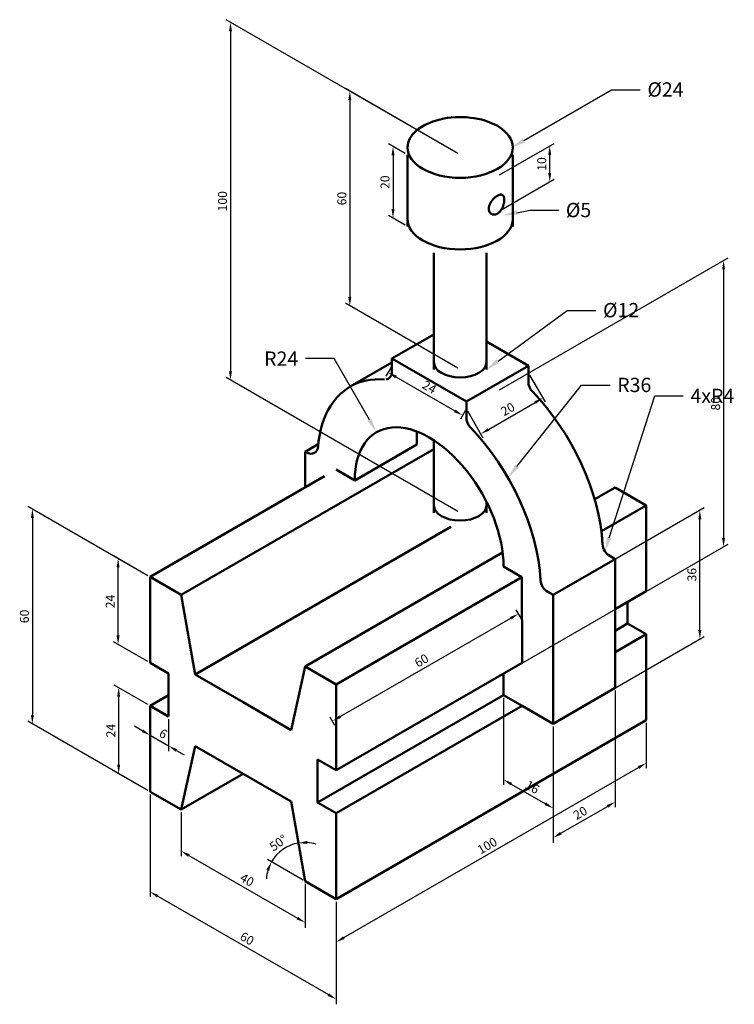
# Model space of a CAD drawing. Units: millimetres. Extents: x 2710 to 2910, y 851 to 1126.
import ezdxf
from ezdxf import colors
from ezdxf.entities.mleader import LeaderData, LeaderLine
from ezdxf.math import Vec2, Vec3

# ---------------------------------------------------------------- set-up
doc = ezdxf.new("R2010")
doc.units = ezdxf.units.MM
for name, color, linetype, lineweight in [('M-DIMS', 2, 'Continuous', 25), ('M-OUTL', 7, 'Continuous', 50), ('M-TEXT', 3, 'Continuous', 25)]:
    doc.layers.add(name, color=color, linetype=linetype, lineweight=lineweight)
doc.styles.get("Standard").update_dxf_attribs({"font": 'arial.ttf'})
doc.dimstyles.new('ISO-25', dxfattribs={"dimtxt": 2.5, "dimasz": 2.5, "dimexe": 1.25, "dimexo": 0.625, "dimtad": 1, "dimtxsty": 'Standard', "dimcen": 2.5, "dimadec": 0, "dimazin": 0, "dimtfac": 1, "dimtmove": 0, "dimatfit": 3, "dimfxl": 1, "dimarcsym": 0})

# ---------------------------------------------------------------- blocks, each defined once
blk = doc.blocks.new('*D1')
at = {"layer": 'Defpoints', "color": 0, "transparency": 16777216}
for p in [(2786.12, 907.33), (2785.15, 894.79), (2790.02, 885.08), (2790.02, 885.08), (2798.68, 880.08)]:
    blk.add_point(p, dxfattribs=at)
at = {"layer": 'M-DIMS', "color": 0, "lineweight": -2, "transparency": 16777216}
blk.add_line((2789.47, 885.4), (2779.53, 891.14), dxfattribs=at)
for start, end in [(99.9347, 150), (73.4842, 86.7094), (163.2252, 176.4505)]:
    blk.add_arc((2790.02, 885.08), 10.85, start, end, dxfattribs=at)
at = {"layer": 'M-DIMS', "color": 0, "transparency": 16777216}
for points in [[(2790.66, 895.5), (2790.61, 896.34), (2788.14, 895.78)], [(2779.24, 888.38), (2780.01, 888.05), (2780.62, 890.51)]]:
    blk.add_solid(points, dxfattribs=at)
at = {"layer": 'M-DIMS', "color": 0, "transparency": 16777216, "insert": (2782.71, 895.54), "char_height": 2.5, "attachment_point": 5, "rotation": 34.9673}
blk.add_mtext('50°', dxfattribs=at)
blk = doc.blocks.new('*D2')
at = {"layer": 'Defpoints', "color": 0, "transparency": 16777216}
for p in [(2885.28, 930.08), (2885.28, 918.09), (2798.68, 880.08)]:
    blk.add_point(p, dxfattribs=at)
at = {"layer": 'M-DIMS', "color": 0, "lineweight": -2, "transparency": 16777216}
for p, q in [((2885.28, 929.36), (2885.28, 916.65)), ((2800.84, 869.34), (2883.11, 916.84)), ((2798.68, 879.36), (2798.68, 866.65))]:
    blk.add_line(p, q, dxfattribs=at)
at = {"layer": 'M-DIMS', "color": 0, "transparency": 16777216}
for points in [[(2882.91, 917.2), (2883.32, 916.48), (2885.28, 918.09)], [(2800.63, 869.7), (2801.05, 868.98), (2798.68, 868.09)]]:
    blk.add_solid(points, dxfattribs=at)
at = {"layer": 'M-DIMS', "color": 0, "transparency": 16777216, "insert": (2841.03, 894.74), "char_height": 2.5, "attachment_point": 5, "rotation": 30}
blk.add_mtext('100', dxfattribs=at)
blk = doc.blocks.new('*D3')
at = {"layer": 'Defpoints', "color": 0, "transparency": 16777216}
for p in [(2737.95, 939.15), (2746.71, 934.08), (2746.71, 910.08)]:
    blk.add_point(p, dxfattribs=at)
at = {"layer": 'M-DIMS', "color": 0, "lineweight": -2, "transparency": 16777216}
for p, q in [((2746.09, 934.44), (2736.7, 939.87)), ((2737.95, 917.65), (2737.95, 936.65)), ((2746.09, 910.44), (2736.7, 915.87))]:
    blk.add_line(p, q, dxfattribs=at)
at = {"layer": 'M-DIMS', "color": 0, "transparency": 16777216}
for points in [[(2737.53, 936.65), (2738.36, 936.65), (2737.95, 939.15)], [(2737.53, 917.65), (2738.36, 917.65), (2737.95, 915.15)]]:
    blk.add_solid(points, dxfattribs=at)
at = {"layer": 'M-DIMS', "color": 0, "transparency": 16777216, "insert": (2736.07, 927.15), "char_height": 2.5, "attachment_point": 5, "rotation": 90}
blk.add_mtext('24', dxfattribs=at)
blk = doc.blocks.new('*D4')
at = {"layer": 'Defpoints', "color": 0, "transparency": 16777216}
for p in [(2737.78, 975.24), (2746.71, 970.08), (2746.71, 946.08)]:
    blk.add_point(p, dxfattribs=at)
at = {"layer": 'M-DIMS', "color": 0, "lineweight": -2, "transparency": 16777216}
for p, q in [((2746.09, 970.44), (2736.53, 975.96)), ((2737.78, 953.74), (2737.78, 972.74)), ((2746.09, 946.44), (2736.53, 951.96))]:
    blk.add_line(p, q, dxfattribs=at)
at = {"layer": 'M-DIMS', "color": 0, "transparency": 16777216}
for points in [[(2737.37, 972.74), (2738.2, 972.74), (2737.78, 975.24)], [(2737.37, 953.74), (2738.2, 953.74), (2737.78, 951.24)]]:
    blk.add_solid(points, dxfattribs=at)
at = {"layer": 'M-DIMS', "color": 0, "transparency": 16777216, "insert": (2735.9, 963.24), "char_height": 2.5, "attachment_point": 5, "rotation": 90}
blk.add_mtext('24', dxfattribs=at)
blk = doc.blocks.new('*D5')
at = {"layer": 'Defpoints', "color": 0, "transparency": 16777216}
for p in [(2746.71, 934.08), (2751.91, 931.08), (2751.91, 922.89)]:
    blk.add_point(p, dxfattribs=at)
at = {"layer": 'M-DIMS', "color": 0, "lineweight": -2, "transparency": 16777216}
for p, q in [((2746.71, 933.36), (2746.71, 924.44)), ((2751.91, 930.36), (2751.91, 921.44)), ((2744.55, 927.14), (2742.38, 928.39)), ((2746.71, 925.89), (2751.91, 922.89)), ((2754.08, 921.64), (2756.24, 920.39))]:
    blk.add_line(p, q, dxfattribs=at)
at = {"layer": 'M-DIMS', "color": 0, "transparency": 16777216}
for points in [[(2744.76, 927.5), (2744.34, 926.78), (2746.71, 925.89)], [(2754.28, 922), (2753.87, 921.28), (2751.91, 922.89)]]:
    blk.add_solid(points, dxfattribs=at)
at = {"layer": 'M-DIMS', "color": 0, "transparency": 16777216, "insert": (2750.26, 926.03), "char_height": 2.5, "attachment_point": 5, "rotation": 330}
blk.add_mtext('6', dxfattribs=at)
blk = doc.blocks.new('*D6')
at = {"layer": 'Defpoints', "color": 0, "transparency": 16777216}
for p in [(2849.63, 959.82), (2850.64, 958.08), (2798.68, 928.08)]:
    blk.add_point(p, dxfattribs=at)
at = {"layer": 'M-DIMS', "color": 0, "lineweight": -2, "transparency": 16777216}
for p, q in [((2850.33, 958.62), (2849.01, 960.91)), ((2799.84, 931.07), (2847.47, 958.57)), ((2798.36, 928.62), (2797.05, 930.91))]:
    blk.add_line(p, q, dxfattribs=at)
at = {"layer": 'M-DIMS', "color": 0, "transparency": 16777216}
for points in [[(2847.26, 958.93), (2847.68, 958.21), (2849.63, 959.82)], [(2799.63, 931.43), (2800.05, 930.71), (2797.67, 929.82)]]:
    blk.add_solid(points, dxfattribs=at)
at = {"layer": 'M-DIMS', "color": 0, "transparency": 16777216, "insert": (2822.7, 946.47), "char_height": 2.5, "attachment_point": 5, "rotation": 30}
blk.add_mtext('60', dxfattribs=at)
blk = doc.blocks.new('*D7')
at = {"layer": 'Defpoints', "color": 0, "transparency": 16777216}
for p in [(2876.62, 939.08), (2859.3, 929.08), (2876.62, 907.25)]:
    blk.add_point(p, dxfattribs=at)
at = {"layer": 'M-DIMS', "color": 0, "lineweight": -2, "transparency": 16777216}
for p, q in [((2876.62, 938.36), (2876.62, 905.8)), ((2859.3, 928.36), (2859.3, 895.8)), ((2861.46, 898.5), (2874.45, 906))]:
    blk.add_line(p, q, dxfattribs=at)
at = {"layer": 'M-DIMS', "color": 0, "transparency": 16777216}
for points in [[(2874.25, 906.36), (2874.66, 905.64), (2876.62, 907.25)], [(2861.25, 898.86), (2861.67, 898.14), (2859.3, 897.25)]]:
    blk.add_solid(points, dxfattribs=at)
at = {"layer": 'M-DIMS', "color": 0, "transparency": 16777216, "insert": (2867.01, 903.89), "char_height": 2.5, "attachment_point": 5, "rotation": 30}
blk.add_mtext('20', dxfattribs=at)
blk = doc.blocks.new('*D8')
at = {"layer": 'Defpoints', "color": 0, "transparency": 16777216}
for p in [(2900.26, 988.73), (2859.3, 965.08), (2859.3, 929.08)]:
    blk.add_point(p, dxfattribs=at)
at = {"layer": 'M-DIMS', "color": 0, "lineweight": -2, "transparency": 16777216}
for p, q in [((2859.92, 965.44), (2901.51, 989.46)), ((2900.26, 955.23), (2900.26, 986.23)), ((2859.92, 929.44), (2901.51, 953.46))]:
    blk.add_line(p, q, dxfattribs=at)
at = {"layer": 'M-DIMS', "color": 0, "transparency": 16777216}
for points in [[(2899.85, 986.23), (2900.68, 986.23), (2900.26, 988.73)], [(2899.85, 955.23), (2900.68, 955.23), (2900.26, 952.73)]]:
    blk.add_solid(points, dxfattribs=at)
at = {"layer": 'M-DIMS', "color": 0, "transparency": 16777216, "insert": (2898.36, 970.73), "char_height": 2.5, "attachment_point": 5, "rotation": 90}
blk.add_mtext('36', dxfattribs=at)
blk = doc.blocks.new('*D9')
at = {"layer": 'Defpoints', "color": 0, "transparency": 16777216}
for p in [(2833.32, 1088.02), (2769.18, 1025.06), (2833.32, 988.02)]:
    blk.add_point(p, dxfattribs=at)
at = {"layer": 'M-DIMS', "color": 0, "lineweight": -2, "transparency": 16777216}
for p, q in [((2832.69, 1088.39), (2767.93, 1125.78)), ((2769.18, 1122.56), (2769.18, 1027.56)), ((2832.69, 988.39), (2767.93, 1025.78))]:
    blk.add_line(p, q, dxfattribs=at)
at = {"layer": 'M-DIMS', "color": 0, "transparency": 16777216}
for points in [[(2768.76, 1122.56), (2769.59, 1122.56), (2769.18, 1125.06)], [(2768.76, 1027.56), (2769.59, 1027.56), (2769.18, 1025.06)]]:
    blk.add_solid(points, dxfattribs=at)
at = {"layer": 'M-DIMS', "color": 0, "transparency": 16777216, "insert": (2767.27, 1075.06), "char_height": 2.5, "attachment_point": 5, "rotation": 90}
blk.add_mtext('100', dxfattribs=at)
blk = doc.blocks.new('*D10')
at = {"layer": 'Defpoints', "color": 0, "transparency": 16777216}
for p in [(2833.32, 1088.02), (2802.51, 1045.81), (2833.32, 1028.02)]:
    blk.add_point(p, dxfattribs=at)
at = {"layer": 'M-DIMS', "color": 0, "lineweight": -2, "transparency": 16777216}
for p, q in [((2832.69, 1088.39), (2801.26, 1106.54)), ((2802.51, 1103.31), (2802.51, 1048.31)), ((2832.69, 1028.39), (2801.26, 1046.54))]:
    blk.add_line(p, q, dxfattribs=at)
at = {"layer": 'M-DIMS', "color": 0, "transparency": 16777216}
for points in [[(2802.09, 1103.31), (2802.92, 1103.31), (2802.51, 1105.81)], [(2802.09, 1048.31), (2802.92, 1048.31), (2802.51, 1045.81)]]:
    blk.add_solid(points, dxfattribs=at)
at = {"layer": 'M-DIMS', "color": 0, "transparency": 16777216, "insert": (2800.6, 1075.81), "char_height": 2.5, "attachment_point": 5, "rotation": 90}
blk.add_mtext('60', dxfattribs=at)
blk = doc.blocks.new('*D11')
at = {"layer": 'Defpoints', "color": 0, "transparency": 16777216}
for p in [(2852.37, 1027.02), (2856.39, 1020.06), (2835.05, 1017.02)]:
    blk.add_point(p, dxfattribs=at)
at = {"layer": 'M-DIMS', "color": 0, "lineweight": -2, "transparency": 16777216}
for p, q in [((2852.68, 1026.48), (2857.02, 1018.98)), ((2841.24, 1011.31), (2854.23, 1018.81)), ((2835.36, 1016.48), (2839.7, 1008.98))]:
    blk.add_line(p, q, dxfattribs=at)
at = {"layer": 'M-DIMS', "color": 0, "transparency": 16777216}
for points in [[(2854.02, 1019.17), (2854.44, 1018.45), (2856.39, 1020.06)], [(2841.03, 1011.67), (2841.45, 1010.95), (2839.07, 1010.06)]]:
    blk.add_solid(points, dxfattribs=at)
at = {"layer": 'M-DIMS', "color": 0, "transparency": 16777216, "insert": (2846.78, 1016.7), "char_height": 2.5, "attachment_point": 5, "rotation": 30}
blk.add_mtext('20', dxfattribs=at)
blk = doc.blocks.new('*D12')
at = {"layer": 'Defpoints', "color": 0, "transparency": 16777216}
for p in [(2814.26, 1029.02), (2834.01, 1015.23), (2835.05, 1017.02)]:
    blk.add_point(p, dxfattribs=at)
at = {"layer": 'M-DIMS', "color": 0, "lineweight": -2, "transparency": 16777216}
for p, q in [((2813.95, 1028.48), (2812.61, 1026.15)), ((2815.4, 1025.98), (2831.85, 1016.48)), ((2834.74, 1016.48), (2833.39, 1014.15))]:
    blk.add_line(p, q, dxfattribs=at)
at = {"layer": 'M-DIMS', "color": 0, "transparency": 16777216}
for points in [[(2815.6, 1026.34), (2815.19, 1025.62), (2813.23, 1027.23)], [(2832.06, 1016.84), (2831.64, 1016.12), (2834.01, 1015.23)]]:
    blk.add_solid(points, dxfattribs=at)
at = {"layer": 'M-DIMS', "color": 0, "transparency": 16777216, "insert": (2824.56, 1022.86), "char_height": 2.5, "attachment_point": 5, "rotation": 330}
blk.add_mtext('24', dxfattribs=at)
blk = doc.blocks.new('*D13')
at = {"layer": 'Defpoints', "color": 0, "transparency": 16777216}
for p in [(2843.71, 1022.02), (2906.89, 978.5), (2843.71, 942.02)]:
    blk.add_point(p, dxfattribs=at)
at = {"layer": 'M-DIMS', "color": 0, "lineweight": -2, "transparency": 16777216}
for p, q in [((2844.33, 1022.39), (2908.14, 1059.22)), ((2906.89, 1056), (2906.89, 981)), ((2844.33, 942.39), (2908.14, 979.22))]:
    blk.add_line(p, q, dxfattribs=at)
at = {"layer": 'M-DIMS', "color": 0, "transparency": 16777216}
for points in [[(2906.47, 1056), (2907.3, 1056), (2906.89, 1058.5)], [(2906.47, 981), (2907.3, 981), (2906.89, 978.5)]]:
    blk.add_solid(points, dxfattribs=at)
at = {"layer": 'M-DIMS', "color": 0, "transparency": 16777216, "insert": (2904.99, 1018.5), "char_height": 2.5, "attachment_point": 5, "rotation": 90}
blk.add_mtext('80', dxfattribs=at)
blk = doc.blocks.new('*D14')
at = {"layer": 'Defpoints', "color": 0, "transparency": 16777216}
for p in [(2845.44, 937.08), (2859.3, 929.08), (2859.3, 905.47)]:
    blk.add_point(p, dxfattribs=at)
at = {"layer": 'M-DIMS', "color": 0, "lineweight": -2, "transparency": 16777216}
for p, q in [((2845.44, 936.36), (2845.44, 912.03)), ((2859.3, 928.36), (2859.3, 904.03)), ((2847.61, 912.22), (2857.13, 906.72))]:
    blk.add_line(p, q, dxfattribs=at)
at = {"layer": 'M-DIMS', "color": 0, "transparency": 16777216}
for points in [[(2847.81, 912.58), (2847.4, 911.86), (2845.44, 913.47)], [(2857.34, 907.08), (2856.92, 906.36), (2859.3, 905.47)]]:
    blk.add_solid(points, dxfattribs=at)
at = {"layer": 'M-DIMS', "color": 0, "transparency": 16777216, "insert": (2853.32, 911.12), "char_height": 2.5, "attachment_point": 5, "rotation": 330}
blk.add_mtext('16', dxfattribs=at)
blk = doc.blocks.new('*D15')
at = {"layer": 'Defpoints', "color": 0, "transparency": 16777216}
for p in [(2746.71, 970.08), (2713.85, 929.06), (2746.71, 910.08)]:
    blk.add_point(p, dxfattribs=at)
at = {"layer": 'M-DIMS', "color": 0, "lineweight": -2, "transparency": 16777216}
for p, q in [((2746.09, 970.44), (2712.6, 989.78)), ((2713.85, 986.56), (2713.85, 931.56)), ((2746.09, 910.44), (2712.6, 929.78))]:
    blk.add_line(p, q, dxfattribs=at)
at = {"layer": 'M-DIMS', "color": 0, "transparency": 16777216}
for points in [[(2713.43, 986.56), (2714.27, 986.56), (2713.85, 989.06)], [(2713.43, 931.56), (2714.27, 931.56), (2713.85, 929.06)]]:
    blk.add_solid(points, dxfattribs=at)
at = {"layer": 'M-DIMS', "color": 0, "transparency": 16777216, "insert": (2711.95, 959.06), "char_height": 2.5, "attachment_point": 5, "rotation": 90}
blk.add_mtext('60', dxfattribs=at)
blk = doc.blocks.new('*D16')
at = {"layer": 'Defpoints', "color": 0, "transparency": 16777216}
for p in [(2746.71, 910.08), (2798.68, 880.08), (2798.68, 852.15)]:
    blk.add_point(p, dxfattribs=at)
at = {"layer": 'M-DIMS', "color": 0, "lineweight": -2, "transparency": 16777216}
for p, q in [((2746.71, 909.36), (2746.71, 880.7)), ((2748.88, 880.9), (2796.51, 853.4)), ((2798.68, 879.36), (2798.68, 850.7))]:
    blk.add_line(p, q, dxfattribs=at)
at = {"layer": 'M-DIMS', "color": 0, "transparency": 16777216}
for points in [[(2749.09, 881.26), (2748.67, 880.54), (2746.71, 882.15)], [(2796.72, 853.76), (2796.3, 853.04), (2798.68, 852.15)]]:
    blk.add_solid(points, dxfattribs=at)
at = {"layer": 'M-DIMS', "color": 0, "transparency": 16777216, "insert": (2773.65, 868.79), "char_height": 2.5, "attachment_point": 5, "rotation": 330}
blk.add_mtext('60', dxfattribs=at)
blk = doc.blocks.new('*D17')
at = {"layer": 'Defpoints', "color": 0, "transparency": 16777216}
for p in [(2755.37, 905.08), (2790.02, 885.08), (2790.02, 873.54)]:
    blk.add_point(p, dxfattribs=at)
at = {"layer": 'M-DIMS', "color": 0, "lineweight": -2, "transparency": 16777216}
for p, q in [((2755.37, 904.36), (2755.37, 892.1)), ((2757.54, 892.29), (2787.85, 874.79)), ((2790.02, 884.36), (2790.02, 872.1))]:
    blk.add_line(p, q, dxfattribs=at)
at = {"layer": 'M-DIMS', "color": 0, "transparency": 16777216}
for points in [[(2757.75, 892.65), (2757.33, 891.93), (2755.37, 893.54)], [(2788.06, 875.15), (2787.64, 874.43), (2790.02, 873.54)]]:
    blk.add_solid(points, dxfattribs=at)
at = {"layer": 'M-DIMS', "color": 0, "transparency": 16777216, "insert": (2773.65, 885.19), "char_height": 2.5, "attachment_point": 5, "rotation": 330}
blk.add_mtext('40', dxfattribs=at)
blk = doc.blocks.new('*D18')
at = {"layer": 'Defpoints', "color": 0, "transparency": 16777216}
for p in [(2818.62, 1088.02), (2814.57, 1070.37), (2818.62, 1068.02)]:
    blk.add_point(p, dxfattribs=at)
at = {"layer": 'M-DIMS', "color": 0, "lineweight": -2, "transparency": 16777216}
for p, q in [((2818, 1088.39), (2813.32, 1091.09)), ((2814.57, 1087.87), (2814.57, 1072.87)), ((2818, 1068.39), (2813.32, 1071.09))]:
    blk.add_line(p, q, dxfattribs=at)
at = {"layer": 'M-DIMS', "color": 0, "transparency": 16777216}
for points in [[(2814.15, 1087.87), (2814.98, 1087.87), (2814.57, 1090.37)], [(2814.15, 1072.87), (2814.98, 1072.87), (2814.57, 1070.37)]]:
    blk.add_solid(points, dxfattribs=at)
at = {"layer": 'M-DIMS', "color": 0, "transparency": 16777216, "insert": (2812.66, 1080.37), "char_height": 2.5, "attachment_point": 5, "rotation": 90}
blk.add_mtext('20', dxfattribs=at)
blk = doc.blocks.new('*D19')
at = {"layer": 'Defpoints', "color": 0, "transparency": 16777216}
for p in [(2858.34, 1090.47), (2843.71, 1082.02), (2843.71, 1072.02)]:
    blk.add_point(p, dxfattribs=at)
at = {"layer": 'M-DIMS', "color": 0, "lineweight": -2, "transparency": 16777216}
for p, q in [((2844.33, 1082.39), (2859.59, 1091.19)), ((2858.34, 1082.97), (2858.34, 1087.97)), ((2844.33, 1072.39), (2859.59, 1081.19))]:
    blk.add_line(p, q, dxfattribs=at)
at = {"layer": 'M-DIMS', "color": 0, "transparency": 16777216}
for points in [[(2857.92, 1087.97), (2858.75, 1087.97), (2858.34, 1090.47)], [(2857.92, 1082.97), (2858.75, 1082.97), (2858.34, 1080.47)]]:
    blk.add_solid(points, dxfattribs=at)
at = {"layer": 'M-DIMS', "color": 0, "transparency": 16777216, "insert": (2856.43, 1085.47), "char_height": 2.5, "attachment_point": 5, "rotation": 90}
blk.add_mtext('10', dxfattribs=at)

msp = doc.modelspace()

# ---------------------------------------------------------------- linework, layer by layer
at = {"layer": 'M-OUTL'}
for p, q in [((2818.62, 1088.025), (2818.62, 1068.025)), ((2848.014, 1088.025), (2848.014, 1068.025)), ((2825.969, 1060.676), (2825.969, 1028.025)), ((2840.666, 1060.676), (2840.666, 1028.025)), ((2814.265, 1031.084), (2825.969, 1037.841)), ((2852.37, 1029.084), (2840.666, 1035.841)), ((2814.265, 1029.995), (2802.612, 1023.267)), ((2835.049, 1019.084), (2814.265, 1031.084)), ((2814.265, 1027.744), (2814.265, 1031.084)), ((2814.265, 1027.075), (2814.265, 1029.025)), ((2835.049, 1019.084), (2852.37, 1029.084)), ((2852.37, 1025.744), (2852.37, 1029.084)), ((2852.37, 1024.669), (2852.37, 1027.025)), ((2835.049, 1015.744), (2835.049, 1019.084)), ((2835.049, 1014.669), (2835.049, 1017.025)), ((2821.193, 1007.084), (2821.193, 1010.748)), ((2790.016, 1005.084), (2793.698, 1007.21)), ((2803.872, 997.084), (2821.193, 1007.084)), ((2825.969, 988.025), (2825.969, 1008.278)), ((2755.375, 965.084), (2825.969, 1005.841)), ((2790.19, 1004.983), (2790.016, 1005.084)), ((2790.016, 995.084), (2790.016, 1005.084)), ((2798.676, 1000.084), (2803.872, 997.084)), ((2746.715, 970.084), (2795.462, 998.228)), ((2870.911, 991.788), (2876.619, 995.084)), ((2885.279, 990.084), (2876.619, 995.084)), ((2840.666, 988.025), (2840.666, 991.148)), ((2885.279, 990.084), (2872.779, 982.867)), ((2885.279, 990.084), (2885.279, 966.084)), ((2759.272, 942.834), (2830.685, 984.064)), ((2790.016, 945.084), (2845.192, 976.939)), ((2859.298, 965.084), (2876.619, 975.084)), ((2875.096, 975.963), (2876.619, 975.084)), ((2876.619, 975.084), (2876.619, 939.084)), ((2850.553, 970.034), (2845.441, 972.985)), ((2746.715, 946.084), (2746.715, 970.084)), ((2746.715, 970.084), (2755.375, 965.084)), ((2850.553, 970.034), (2798.676, 940.084)), ((2850.638, 946.084), (2850.553, 970.034)), ((2859.298, 965.084), (2857.775, 965.963)), ((2876.619, 961.084), (2885.279, 966.084)), ((2755.375, 965.084), (2759.272, 942.834)), ((2859.298, 929.084), (2859.298, 965.084)), ((2880.083, 963.084), (2880.083, 957.084)), ((2876.619, 955.084), (2880.083, 957.084)), ((2880.083, 957.084), (2885.279, 954.084)), ((2876.619, 949.084), (2885.279, 954.084)), ((2885.279, 954.084), (2885.279, 930.084)), ((2751.911, 943.084), (2746.715, 946.084)), ((2786.119, 927.334), (2790.016, 945.084)), ((2798.676, 940.084), (2790.016, 945.084)), ((2798.676, 916.084), (2850.638, 946.084)), ((2798.676, 916.084), (2850.638, 946.084)), ((2751.911, 931.084), (2751.911, 943.084)), ((2772.695, 935.084), (2759.272, 942.834)), ((2845.442, 937.084), (2845.442, 943.084)), ((2798.676, 940.084), (2798.676, 916.084)), ((2876.619, 939.084), (2859.298, 929.084)), ((2746.715, 934.084), (2751.911, 937.084)), ((2793.48, 907.084), (2845.442, 937.084)), ((2850.638, 934.084), (2845.442, 937.084)), ((2746.715, 910.084), (2746.715, 934.084)), ((2746.715, 934.084), (2751.911, 931.084)), ((2772.695, 935.084), (2786.119, 927.334)), ((2798.676, 904.084), (2850.638, 934.084)), ((2798.676, 904.084), (2850.638, 934.084)), ((2850.638, 934.084), (2859.298, 929.084)), ((2798.676, 880.084), (2885.279, 930.084)), ((2759.272, 922.834), (2755.375, 905.084)), ((2772.695, 915.084), (2759.272, 922.834)), ((2798.676, 916.084), (2793.48, 919.084)), ((2793.48, 919.084), (2793.48, 907.084)), ((2755.375, 905.084), (2772.695, 915.084)), ((2772.695, 915.084), (2786.119, 907.334)), ((2746.715, 910.084), (2755.375, 905.084)), ((2786.119, 907.334), (2790.016, 885.084)), ((2793.48, 907.084), (2798.676, 904.084)), ((2798.676, 904.084), (2798.676, 880.084)), ((2798.676, 880.084), (2790.016, 885.084))]:
    msp.add_line(p, q, dxfattribs=at)
for points in [[(2842.065, 1071.497), (2842.026, 1071.521), (2841.988, 1071.546), (2841.951, 1071.572), (2841.914, 1071.599), (2841.878, 1071.628), (2841.843, 1071.657), (2841.81, 1071.688), (2841.777, 1071.721), (2841.745, 1071.754), (2841.714, 1071.789), (2841.684, 1071.825), (2841.655, 1071.862), (2841.627, 1071.9), (2841.6, 1071.939), (2841.575, 1071.979), (2841.55, 1072.02), (2841.527, 1072.062), (2841.504, 1072.105), (2841.483, 1072.149), (2841.463, 1072.194), (2841.445, 1072.24), (2841.427, 1072.287), (2841.411, 1072.335), (2841.396, 1072.383), (2841.382, 1072.432), (2841.37, 1072.483), (2841.359, 1072.533), (2841.349, 1072.585), (2841.34, 1072.637), (2841.333, 1072.69), (2841.327, 1072.743), (2841.323, 1072.798), (2841.319, 1072.852), (2841.317, 1072.908), (2841.316, 1072.963), (2841.317, 1073.02), (2841.319, 1073.076), (2841.322, 1073.134), (2841.327, 1073.191), (2841.333, 1073.249), (2841.34, 1073.308), (2841.348, 1073.367), (2841.358, 1073.426), (2841.369, 1073.486), (2841.382, 1073.546), (2841.396, 1073.606), (2841.411, 1073.667), (2841.427, 1073.728), (2841.445, 1073.789), (2841.464, 1073.85), (2841.485, 1073.912), (2841.507, 1073.974), (2841.53, 1074.037), (2841.554, 1074.099), (2841.58, 1074.162), (2841.607, 1074.225), (2841.635, 1074.288), (2841.665, 1074.352), (2841.696, 1074.415), (2841.729, 1074.479), (2841.762, 1074.543), (2841.798, 1074.607), (2841.834, 1074.671), (2841.872, 1074.735), (2841.911, 1074.799), (2841.951, 1074.863), (2841.993, 1074.927), (2842.036, 1074.991), (2842.081, 1075.055), (2842.127, 1075.12), (2842.175, 1075.184), (2842.224, 1075.249), (2842.274, 1075.313), (2842.326, 1075.377), (2842.379, 1075.441), (2842.434, 1075.505), (2842.49, 1075.568), (2842.547, 1075.631), (2842.605, 1075.693), (2842.664, 1075.755), (2842.725, 1075.815), (2842.786, 1075.875), (2842.848, 1075.934), (2842.911, 1075.992), (2842.975, 1076.049), (2843.04, 1076.105), (2843.105, 1076.16), (2843.171, 1076.213), (2843.237, 1076.265), (2843.304, 1076.315), (2843.371, 1076.364), (2843.438, 1076.412), (2843.506, 1076.457), (2843.574, 1076.501), (2843.642, 1076.543), (2843.71, 1076.584)], [(2845.127, 1076.801), (2845.168, 1076.776), (2845.206, 1076.748), (2845.243, 1076.719), (2845.277, 1076.687), (2845.31, 1076.653), (2845.342, 1076.616), (2845.371, 1076.578), (2845.399, 1076.538), (2845.425, 1076.496), (2845.45, 1076.452), (2845.473, 1076.406), (2845.495, 1076.359), (2845.515, 1076.309), (2845.533, 1076.258), (2845.55, 1076.206), (2845.566, 1076.151), (2845.58, 1076.096), (2845.593, 1076.038), (2845.604, 1075.98), (2845.614, 1075.919), (2845.623, 1075.858), (2845.63, 1075.795), (2845.636, 1075.73), (2845.641, 1075.665), (2845.644, 1075.598), (2845.646, 1075.529), (2845.647, 1075.46), (2845.646, 1075.389), (2845.644, 1075.318), (2845.64, 1075.245), (2845.635, 1075.171), (2845.629, 1075.096), (2845.622, 1075.02), (2845.613, 1074.943), (2845.603, 1074.865), (2845.591, 1074.786), (2845.578, 1074.706), (2845.564, 1074.625), (2845.548, 1074.544), (2845.531, 1074.462), (2845.512, 1074.379), (2845.492, 1074.295), (2845.47, 1074.211), (2845.447, 1074.126), (2845.422, 1074.04), (2845.395, 1073.954), (2845.367, 1073.867), (2845.337, 1073.78), (2845.306, 1073.693), (2845.272, 1073.605), (2845.237, 1073.517), (2845.201, 1073.429), (2845.162, 1073.341), (2845.121, 1073.253), (2845.079, 1073.165), (2845.035, 1073.077), (2844.988, 1072.99), (2844.939, 1072.902), (2844.888, 1072.814), (2844.834, 1072.726), (2844.777, 1072.638), (2844.718, 1072.551), (2844.657, 1072.465), (2844.593, 1072.381), (2844.527, 1072.298), (2844.458, 1072.217), (2844.388, 1072.138), (2844.316, 1072.062), (2844.241, 1071.988), (2844.165, 1071.917), (2844.088, 1071.85), (2844.008, 1071.786), (2843.928, 1071.725), (2843.846, 1071.668), (2843.763, 1071.615), (2843.679, 1071.566), (2843.595, 1071.522), (2843.51, 1071.481), (2843.425, 1071.445), (2843.339, 1071.413), (2843.254, 1071.385), (2843.168, 1071.362), (2843.084, 1071.343), (2842.999, 1071.329), (2842.915, 1071.319), (2842.832, 1071.314), (2842.749, 1071.313), (2842.667, 1071.316), (2842.587, 1071.324), (2842.507, 1071.336), (2842.429, 1071.353), (2842.353, 1071.373), (2842.278, 1071.398), (2842.205, 1071.427), (2842.134, 1071.46), (2842.065, 1071.497)], [(2843.71, 1076.584), (2843.729, 1076.595), (2843.748, 1076.606), (2843.767, 1076.616), (2843.786, 1076.627), (2843.805, 1076.637), (2843.824, 1076.647), (2843.843, 1076.657), (2843.862, 1076.667), (2843.881, 1076.676), (2843.9, 1076.685), (2843.918, 1076.695), (2843.937, 1076.703), (2843.955, 1076.712), (2843.973, 1076.721), (2843.992, 1076.729), (2844.01, 1076.737), (2844.028, 1076.745), (2844.046, 1076.753), (2844.064, 1076.76), (2844.081, 1076.768), (2844.099, 1076.775), (2844.117, 1076.782), (2844.134, 1076.789), (2844.152, 1076.795), (2844.169, 1076.802), (2844.186, 1076.808), (2844.204, 1076.814), (2844.221, 1076.82), (2844.238, 1076.825), (2844.254, 1076.831), (2844.271, 1076.836), (2844.288, 1076.841), (2844.304, 1076.846), (2844.321, 1076.85), (2844.337, 1076.855), (2844.354, 1076.859), (2844.37, 1076.863), (2844.386, 1076.867), (2844.402, 1076.871), (2844.418, 1076.874), (2844.433, 1076.878), (2844.449, 1076.881), (2844.464, 1076.884), (2844.48, 1076.887), (2844.495, 1076.889), (2844.51, 1076.892), (2844.525, 1076.894), (2844.54, 1076.896), (2844.555, 1076.898), (2844.57, 1076.899), (2844.585, 1076.901), (2844.599, 1076.902), (2844.614, 1076.903), (2844.628, 1076.904), (2844.642, 1076.905), (2844.656, 1076.906), (2844.67, 1076.906), (2844.684, 1076.907), (2844.698, 1076.907), (2844.712, 1076.907), (2844.725, 1076.907), (2844.739, 1076.906), (2844.752, 1076.906), (2844.765, 1076.905), (2844.778, 1076.904), (2844.791, 1076.903), (2844.804, 1076.902), (2844.817, 1076.9), (2844.83, 1076.899), (2844.842, 1076.897), (2844.854, 1076.895), (2844.867, 1076.893), (2844.879, 1076.891), (2844.891, 1076.889), (2844.903, 1076.886), (2844.915, 1076.884), (2844.926, 1076.881), (2844.938, 1076.878), (2844.95, 1076.875), (2844.961, 1076.872), (2844.972, 1076.868), (2844.983, 1076.865), (2844.994, 1076.861), (2845.005, 1076.857), (2845.016, 1076.853), (2845.027, 1076.849), (2845.037, 1076.845), (2845.048, 1076.84), (2845.058, 1076.836), (2845.068, 1076.831), (2845.078, 1076.826), (2845.088, 1076.822), (2845.098, 1076.817), (2845.108, 1076.811), (2845.118, 1076.806), (2845.127, 1076.801)]]:
    msp.add_lwpolyline(points, dxfattribs=at)
for centre, start, end in [((2856.37, 1024.669), 180, 223.98051), ((2839.049, 1014.669), 180, 223.98051), ((2877.096, 979.427), 182.83372, 240), ((2859.775, 969.427), 182.83372, 240)]:
    msp.add_arc(centre, 4, start, end, dxfattribs=at)
for centre, major_axis, start_param, end_param in [((2833.317, 1090.084), (14.697, 0), 0.7853982, 3.1415927), ((2833.317, 1090.084), (14.697, 0), 0, 0.7853982), ((2833.317, 1090.084), (14.697, 0), 3.1415927, 6.2831853), ((2833.317, 1070.084), (14.697, 0), 3.1415927, 6.2831853), ((2833.317, 1030.084), (7.348, 0), 3.1415927, 6.2831853), ((2811.493, 1029.498), (1.531, -4.18), 6.1460382, 7.0428047), ((2824.657, 985.084), (-22.045, 38.184), 5.909304, 6.2831853), ((2824.657, 985.084), (-22.045, 38.184), 0, 0.6852307), ((2841.977, 995.084), (22.045, -38.184), 0.8441674, 1.9779262), ((2824.657, 985.084), (14.697, -25.456), 0.7813003, 3.9269908), ((2824.657, 985.084), (22.045, -38.184), 0.8441674, 1.9779262), ((2790.19, 1008.983), (2.449, -4.243), 5.4977871, 6.2831853), ((2790.19, 1008.983), (2.449, -4.243), 0, 0.6852307), ((2833.317, 990.084), (7.348, 0), 3.1415927, 6.2831853)]:
    msp.add_ellipse(centre, major_axis=major_axis, ratio=0.5773503, start_param=start_param, end_param=end_param, dxfattribs=at)

# ---------------------------------------------------------------- dimensions: what is measured, and where the dimension line sits
at = {"layer": 'M-DIMS'}
for p1, p2, distance, picture, middle in [((2833.317, 1088.025), (2833.317, 988.025), -64.141, '*D9', (2767.275, 1075.057)), ((2833.317, 1088.025), (2833.317, 1028.025), -30.812, '*D10', (2800.604, 1075.814)), ((2814.265, 1029.025), (2835.049, 1017.025), -2.069, '*D12', (2824.563, 1022.861)), ((2835.049, 1017.025), (2852.37, 1027.025), -8.045, '*D11', (2846.781, 1016.704)), ((2746.715, 970.084), (2746.715, 910.084), -32.866, '*D15', (2711.948, 959.059)), ((2859.298, 929.084), (2859.298, 965.084), -40.965, '*D8', (2898.36, 970.735)), ((2746.715, 946.084), (2746.715, 970.084), 8.93, '*D4', (2735.905, 963.239)), ((2798.676, 928.084), (2850.638, 958.084), 2.008, '*D6', (2822.702, 946.47)), ((2746.715, 910.084), (2746.715, 934.084), 8.768, '*D3', (2736.066, 927.146)), ((2859.298, 929.084), (2876.619, 939.084), -27.572, '*D7', (2867.008, 903.893)), ((2845.442, 937.084), (2859.298, 929.084), -20.448, '*D14', (2853.321, 911.119)), ((2746.715, 934.084), (2751.911, 931.084), -7.099, '*D5', (2750.263, 926.033)), ((2798.676, 880.084), (2885.279, 930.084), -10.385, '*D2', (2841.027, 894.739)), ((2746.715, 910.084), (2798.676, 880.084), -24.193, '*D16', (2773.646, 868.794)), ((2755.375, 905.084), (2790.016, 885.084), -9.994, '*D17', (2773.646, 885.19))]:
    dim = msp.add_aligned_dim(p1=p1, p2=p2, distance=distance, dimstyle='ISO-25', override={"dimclrd": 0, "dimclre": 0, "dimclrt": 0}, dxfattribs=at)
    dim.commit()
    dim.dimension.update_dxf_attribs({"geometry": picture, "text_midpoint": middle})
for base, p1, p2, picture, middle in [((2814.566, 1070.365), (2818.62, 1088.025), (2818.62, 1068.025), '*D18', (2812.665, 1080.365)), ((2858.335, 1090.469), (2843.71, 1072.025), (2843.71, 1082.025), '*D19', (2856.434, 1085.469)), ((2906.887, 978.5), (2843.71, 1022.025), (2843.71, 942.025), '*D13', (2904.986, 1018.5))]:
    dim = msp.add_linear_dim(base=base, p1=p1, p2=p2, angle=90, dimstyle='ISO-25', override={"dimclrd": 0, "dimclre": 0, "dimclrt": 0}, dxfattribs=at)
    dim.commit()
    dim.dimension.update_dxf_attribs({"geometry": picture, "text_midpoint": middle})
dim = msp.add_angular_dim_2l(base=(2785.152, 894.788), line1=((2786.119, 907.334), (2790.016, 885.084)), line2=((2798.676, 880.084), (2790.016, 885.084)), dimstyle='ISO-25', override={"dimclrd": 0, "dimclre": 0, "dimclrt": 0}, dxfattribs=at)
dim.commit()
dim.dimension.update_dxf_attribs({"geometry": '*D1', "text_midpoint": (2782.705, 895.537)})

# ---------------------------------------------------------------- leaders
at = {"layer": 'M-TEXT'}
ml = msp.add_multileader_mtext('Standard', dxfattribs=at)
ml.set_content('%%C24', color=256)
ml.set_leader_properties()
ml.build(insert=Vec2(0, 0))
ctx = ml.context
ctx.base_point, ctx.plane_origin = Vec3(2883.622, 1106.203), Vec3(2847.6, 1090.025)
notes = []
notes.append((ctx, [(0, (1, 1, 0), (2875.622, 1106.203), (1, 0), 8, [(0, [(2847.6, 1090.025)], 0, [])])]))
ctx.mtext.insert, ctx.mtext.flow_direction = Vec3(2885.622, 1108.284), 5
ml = msp.add_multileader_mtext('Standard', dxfattribs=at)
ml.set_content('%%C5', color=256)
ml.set_leader_properties()
ml.build(insert=Vec2(0, 0))
ctx = ml.context
ctx.base_point, ctx.plane_origin = Vec3(2860.842, 1072.52), Vec3(2845.24, 1071.141)
notes.append((ctx, [(0, (1, 1, 0), (2852.842, 1072.52), (1, 0), 8, [(0, [(2845.24, 1071.141)], 0, [])])]))
ctx.mtext.insert, ctx.mtext.flow_direction = Vec3(2862.842, 1074.6), 5
ml = msp.add_multileader_mtext('Standard', dxfattribs=at)
ml.set_content('%%C12', color=256)
ml.set_leader_properties()
ml.build(insert=Vec2(0, 0))
ctx = ml.context
ctx.base_point, ctx.plane_origin = Vec3(2871.225, 1044.553), Vec3(2840.666, 1028.025)
notes.append((ctx, [(0, (1, 1, 0), (2863.225, 1044.553), (1, 0), 8, [(0, [(2840.666, 1028.025)], 0, [])])]))
ctx.mtext.insert, ctx.mtext.flow_direction = Vec3(2873.225, 1046.634), 5
ml = msp.add_multileader_mtext('Standard', dxfattribs=at)
ml.set_content('R24', color=256)
ml.set_leader_properties()
ml.build(insert=Vec2(0, 0))
ctx = ml.context
ctx.base_point, ctx.plane_origin = Vec3(2776.557, 1031.084), Vec3(2809.96, 1010.539)
ctx.text_align_type = 2
notes.append((ctx, [(0, (1, 1, 0), (2798.098, 1031.084), (-1, 0), 8, [(0, [(2809.96, 1010.539)], 0, [])])]))
ctx.mtext.insert, ctx.mtext.alignment, ctx.mtext.flow_direction = Vec3(2788.098, 1033.084), 3, 5
ml = msp.add_multileader_mtext('Standard', dxfattribs=at)
ml.set_content('R36', color=256)
ml.set_leader_properties()
ml.build(insert=Vec2(0, 0))
ctx = ml.context
ctx.base_point, ctx.plane_origin = Vec3(2875.183, 1023.708), Vec3(2846.702, 997.812)
notes.append((ctx, [(0, (1, 1, 0), (2867.183, 1023.708), (1, 0), 8, [(0, [(2846.702, 997.812)], 0, [])])]))
ctx.mtext.insert, ctx.mtext.flow_direction = Vec3(2877.183, 1025.743), 5
ml = msp.add_multileader_mtext('Standard', dxfattribs=at)
ml.set_content('4xR4', color=256)
ml.set_leader_properties()
ml.build(insert=Vec2(0, 0))
ctx = ml.context
ctx.base_point, ctx.plane_origin = Vec3(2895.646, 1020.669), Vec3(2873.748, 977.238)
notes.append((ctx, [(0, (1, 1, 0), (2887.646, 1020.669), (1, 0), 8, [(0, [(2873.748, 977.238)], 0, [])])]))
ctx.mtext.insert, ctx.mtext.flow_direction = Vec3(2897.646, 1022.669), 5
for ctx, leaders in notes:
    for number, flags, end, landing, length, lines in leaders:
        leader = LeaderData()
        leader.index, (leader.has_last_leader_line, leader.has_dogleg_vector, leader.attachment_direction) = number, flags
        leader.last_leader_point, leader.dogleg_vector, leader.dogleg_length = Vec3(end), Vec3(landing), length
        for number, points, colour, breaks in lines:
            line = LeaderLine()
            line.index, line.vertices, line.color, line.breaks = number, Vec3.list(points), colors.encode_raw_color(colour), breaks
            leader.lines.append(line)
        ctx.leaders.append(leader)

doc.saveas('drawing.dxf')
